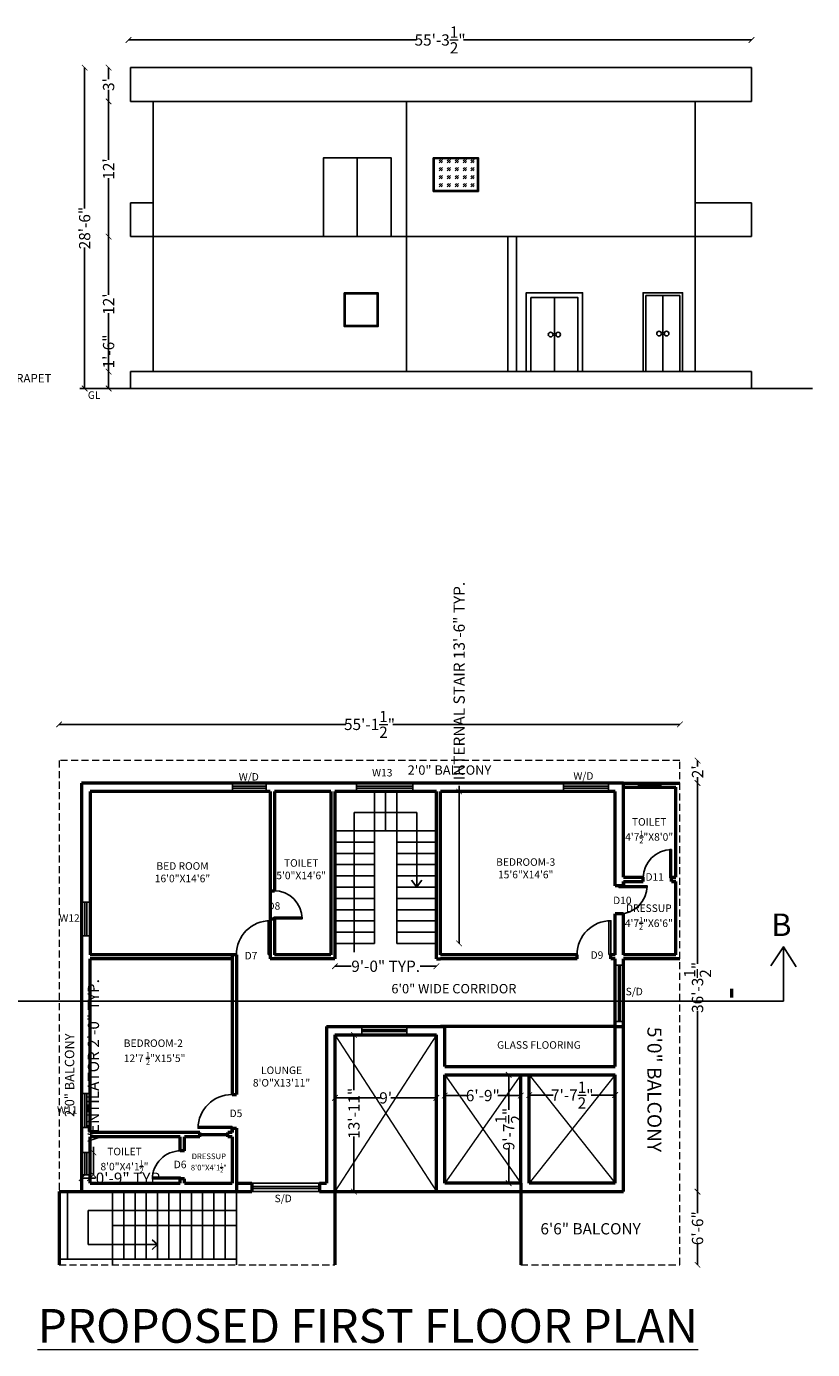
# Model space of a CAD drawing. Units: inches. Extents: x 626 to 5030, y -1681 to 1720.
# Tile 4 of 5: x 3160 to 3997, y 310 to 1720. Entities that reach past the tile are written whole.
import ezdxf
from ezdxf import colors
from ezdxf.entities.mleader import LeaderData, LeaderLine
from ezdxf.math import Vec2, Vec3

# ---------------------------------------------------------------- set-up
doc = ezdxf.new("R2010")
doc.units = ezdxf.units.IN
doc.header["$MEASUREMENT"] = 0
doc.linetypes.add('HIDDENX2', pattern=[0.75, 0.5, -0.25])
for name, color, linetype, lineweight in [('A-ANNO-DIMS', 2, 'Continuous', 18), ('A-ANNO-SYMB', 2, 'Continuous', 25), ('A-ANNO-TEXT', 7, 'Continuous', 18), ('A-AREA-IDEN', 3, 'Continuous', 18), ('A-DOOR', 4, 'Continuous', 25), ('A-ELEV', 7, 'Continuous', 25), ('A-FLOR-OVHD', 3, 'HIDDENX2', 18), ('A-FLOR-PATT', 8, 'Continuous', 18), ('A-FLOR-STRS', 3, 'Continuous', 25), ('A-GLAZ', 4, 'Continuous', 25), ('A-WALL', 7, 'Continuous', 50)]:
    doc.layers.add(name, color=color, linetype=linetype, lineweight=lineweight)
doc.layers.add('windows', color=4, linetype='Continuous')
doc.styles.get("Standard").update_dxf_attribs({"font": 'arial.ttf'})
doc.dimstyles.get("Standard").update_dxf_attribs({"dimtxt": 12, "dimasz": 6, "dimexe": 0.18, "dimexo": 0.0625, "dimgap": 0.09, "dimtad": 0, "dimdec": 1, "dimzin": 0, "dimdsep": 46, "dimlunit": 4, "dimtxsty": 'Standard', "dimblk": 'ARCHTICK', "dimcen": 0.09, "dimse1": 1, "dimse2": 1, "dimclrt": 3, "dimadec": 0, "dimazin": 0, "dimtfac": 1, "dimtdec": 1, "dimtofl": 0, "dimtmove": 0, "dimatfit": 3, "dimfxl": 1, "dimtolj": 1, "dimtzin": 0, "dimarcsym": 0})

# ---------------------------------------------------------------- blocks, each defined once
blk = doc.blocks.new('*U22')
for p, q in [((-750, 0), (-750, -100)), ((0, 0), (0, -100))]:
    blk.add_line(p, q)
blk.add_lwpolyline([(0, 0), (0, 750), (-43.75, 750), (-43.75, 0)], close=True)
blk.add_arc((0, 0), 750, 90, 180)
blk = doc.blocks.new('W3')
at = {"layer": 'windows'}
for p, q in [((2120.1, 414.9), (2120.1, 378.9)), ((2122.1, 414.9), (2122.1, 378.9))]:
    blk.add_line(p, q, dxfattribs=at)
blk.add_lwpolyline([(2116.6, 414.9), (2125.6, 414.9), (2125.6, 378.9), (2116.6, 378.9)], close=True, dxfattribs=at)
blk = doc.blocks.new('W5')
at = {"layer": 'windows'}
for p, q in [((2038.2, 554.9), (2038.2, 494.9)), ((2040.2, 554.9), (2040.2, 494.9))]:
    blk.add_line(p, q, dxfattribs=at)
blk.add_lwpolyline([(2034.7, 554.9), (2043.7, 554.9), (2043.7, 494.9), (2034.7, 494.9)], close=True, dxfattribs=at)
blk = doc.blocks.new('WINDOW')
at = {"layer": 'windows'}
for p, q in [((173.6, 537.5), (173.6, 489.5)), ((175.6, 537.5), (175.6, 489.5))]:
    blk.add_line(p, q, dxfattribs=at)
blk.add_lwpolyline([(170.1, 537.5), (179.1, 537.5), (179.1, 489.5), (170.1, 489.5)], close=True, dxfattribs=at)
blk = doc.blocks.new('*U21')
for p, q in [((0, 0), (0, -100)), ((750, 0), (750, -100))]:
    blk.add_line(p, q)
blk.add_lwpolyline([(0, 0), (0, 750), (43.75, 750), (43.75, 0)], close=True)
blk.add_arc((0, 0), 750, 0, 90)
blk = doc.blocks.new('*U27')
for p, q in [((0, 0), (0, 100)), ((750, 0), (750, 100))]:
    blk.add_line(p, q)
blk.add_lwpolyline([(0, 0), (0, -750), (43.75, -750), (43.75, 0)], close=True)
blk.add_arc((0, 0), 750, 270, 0)
blk = doc.blocks.new('*U28')
for p, q in [((0, 0), (0, -100)), ((750, 0), (750, -100))]:
    blk.add_line(p, q)
blk.add_lwpolyline([(0, 0), (0, 750), (43.75, 750), (43.75, 0)], close=True)
blk.add_arc((0, 0), 750, 0, 90)
blk = doc.blocks.new('_ArchTick')
at = {"color": 0, "linetype": 'ByBlock', "const_width": 0.15}
blk.add_lwpolyline([(-0.5, -0.5), (0.5, 0.5)], dxfattribs=at)
blk = doc.blocks.new('*D29')
at = {"layer": 'A-ANNO-DIMS', "color": 0, "lineweight": -2, "transparency": 16777216}
for p, q in [((3488.3, 578.4), (3536.7, 578.4)), ((3596.3, 578.4), (3547.9, 578.4))]:
    blk.add_line(p, q, dxfattribs=at)
at = {"layer": 'DEFPOINTS', "color": 0, "transparency": 16777216}
for p in [(3596.3, 578.4), (3488.3, 575.4), (3596.3, 562)]:
    blk.add_point(p, dxfattribs=at)
at = {"layer": 'A-ANNO-DIMS', "color": 0, "lineweight": -2, "transparency": 16777216, "xscale": 6, "yscale": 6, "zscale": 6, "rotation": 180}
blk.add_blockref('_ArchTick', (3488.3, 578.4), dxfattribs=at)
at = {"layer": 'A-ANNO-DIMS', "color": 0, "lineweight": -2, "transparency": 16777216, "xscale": 6, "yscale": 6, "zscale": 6}
blk.add_blockref('_ArchTick', (3596.3, 578.4), dxfattribs=at)
at = {"layer": 'A-ANNO-DIMS', "color": 0, "transparency": 16777216, "insert": (3542.3, 578.4), "char_height": 12, "attachment_point": 5}
blk.add_mtext("\\A1;9'", dxfattribs=at)
blk = doc.blocks.new('*D30')
at = {"layer": 'A-ANNO-DIMS', "color": 0, "lineweight": -2, "transparency": 16777216}
for p, q in [((3508.5, 645.5), (3508.5, 586.8)), ((3508.5, 478.5), (3508.5, 537.2))]:
    blk.add_line(p, q, dxfattribs=at)
at = {"layer": 'DEFPOINTS', "color": 0, "transparency": 16777216}
for p in [(3582, 645.5), (3508.5, 478.5), (3582, 478.5)]:
    blk.add_point(p, dxfattribs=at)
at = {"layer": 'A-ANNO-DIMS', "color": 0, "lineweight": -2, "transparency": 16777216, "xscale": 6, "yscale": 6, "zscale": 6}
for p, rotation in [((3508.5, 645.5), 90), ((3508.5, 478.5), 270)]:
    blk.add_blockref('_ArchTick', p, dxfattribs=dict(at, rotation=rotation))
at = {"layer": 'A-ANNO-DIMS', "color": 0, "transparency": 16777216, "insert": (3508.5, 562), "char_height": 12, "attachment_point": 5, "rotation": 90}
blk.add_mtext('\\A1;13\'-11"', dxfattribs=at)
blk = doc.blocks.new('*D31')
at = {"layer": 'A-ANNO-DIMS', "color": 0, "lineweight": -2, "transparency": 16777216}
for p, q in [((3605.3, 580.9), (3629.7, 580.9)), ((3686.3, 580.9), (3661.9, 580.9))]:
    blk.add_line(p, q, dxfattribs=at)
at = {"layer": 'DEFPOINTS', "color": 0, "transparency": 16777216}
for p in [(3605.3, 603), (3686.3, 603), (3686.3, 580.9)]:
    blk.add_point(p, dxfattribs=at)
at = {"layer": 'A-ANNO-DIMS', "color": 0, "lineweight": -2, "transparency": 16777216, "xscale": 6, "yscale": 6, "zscale": 6, "rotation": 180}
blk.add_blockref('_ArchTick', (3605.3, 580.9), dxfattribs=at)
at = {"layer": 'A-ANNO-DIMS', "color": 0, "lineweight": -2, "transparency": 16777216, "xscale": 6, "yscale": 6, "zscale": 6}
blk.add_blockref('_ArchTick', (3686.3, 580.9), dxfattribs=at)
at = {"layer": 'A-ANNO-DIMS', "color": 0, "transparency": 16777216, "insert": (3645.8, 580.9), "char_height": 12, "attachment_point": 5}
blk.add_mtext('\\A1;6\'-9"', dxfattribs=at)
blk = doc.blocks.new('*D32')
at = {"layer": 'A-ANNO-DIMS', "color": 0, "lineweight": -2, "transparency": 16777216}
for p, q in [((3695.3, 581.4), (3720.7, 581.4)), ((3786.8, 581.4), (3761.4, 581.4))]:
    blk.add_line(p, q, dxfattribs=at)
at = {"layer": 'DEFPOINTS', "color": 0, "transparency": 16777216}
for p in [(3695.3, 603), (3786.8, 603), (3786.8, 581.4)]:
    blk.add_point(p, dxfattribs=at)
at = {"layer": 'A-ANNO-DIMS', "color": 0, "lineweight": -2, "transparency": 16777216, "xscale": 6, "yscale": 6, "zscale": 6, "rotation": 180}
blk.add_blockref('_ArchTick', (3695.3, 581.4), dxfattribs=at)
at = {"layer": 'A-ANNO-DIMS', "color": 0, "lineweight": -2, "transparency": 16777216, "xscale": 6, "yscale": 6, "zscale": 6}
blk.add_blockref('_ArchTick', (3786.8, 581.4), dxfattribs=at)
at = {"layer": 'A-ANNO-DIMS', "color": 0, "transparency": 16777216, "insert": (3741.1, 581.4), "char_height": 12, "attachment_point": 5}
blk.add_mtext('\\A1;7\'-7{\\H1x;\\S1/2;}"', dxfattribs=at)
blk = doc.blocks.new('*D33')
at = {"layer": 'A-ANNO-DIMS', "color": 0, "lineweight": -2, "transparency": 16777216}
for p, q in [((3673.4, 603), (3673.4, 565.7)), ((3673.4, 487.5), (3673.4, 524.8))]:
    blk.add_line(p, q, dxfattribs=at)
at = {"layer": 'DEFPOINTS', "color": 0, "transparency": 16777216}
for p in [(3645.8, 603), (3662, 487.5), (3673.4, 487.5)]:
    blk.add_point(p, dxfattribs=at)
at = {"layer": 'A-ANNO-DIMS', "color": 0, "lineweight": -2, "transparency": 16777216, "xscale": 6, "yscale": 6, "zscale": 6}
for p, rotation in [((3673.4, 603), 90), ((3673.4, 487.5), 270)]:
    blk.add_blockref('_ArchTick', p, dxfattribs=dict(at, rotation=rotation))
at = {"layer": 'A-ANNO-DIMS', "color": 0, "transparency": 16777216, "insert": (3673.4, 545.2), "char_height": 12, "attachment_point": 5, "rotation": 90}
blk.add_mtext('\\A1;9\'-7{\\H1x;\\S1/2;}"', dxfattribs=at)
blk = doc.blocks.new('V1')
at = {"layer": 'windows'}
for p, q in [((3301.5, 317.5), (3301.5, 293.5)), ((3303.5, 317.5), (3303.5, 293.5))]:
    blk.add_line(p, q, dxfattribs=at)
blk.add_lwpolyline([(3298, 317.5), (3307, 317.5), (3307, 293.5), (3298, 293.5)], close=True, dxfattribs=at)
blk = doc.blocks.new('*D35')
at = {"layer": 'A-ANNO-DIMS', "color": 0, "lineweight": -2, "transparency": 16777216}
for p, q in [((3194.3, 976.5), (3500, 976.5)), ((3855.8, 976.5), (3550.1, 976.5))]:
    blk.add_line(p, q, dxfattribs=at)
at = {"layer": 'DEFPOINTS', "color": 0, "transparency": 16777216}
for p in [(3194.3, 976.5), (3194.3, 938), (3855.8, 938)]:
    blk.add_point(p, dxfattribs=at)
at = {"layer": 'A-ANNO-DIMS', "color": 0, "lineweight": -2, "transparency": 16777216, "xscale": 6, "yscale": 6, "zscale": 6, "rotation": 180}
blk.add_blockref('_ArchTick', (3194.3, 976.5), dxfattribs=at)
at = {"layer": 'A-ANNO-DIMS', "color": 0, "lineweight": -2, "transparency": 16777216, "xscale": 6, "yscale": 6, "zscale": 6}
blk.add_blockref('_ArchTick', (3855.8, 976.5), dxfattribs=at)
at = {"layer": 'A-ANNO-DIMS', "color": 0, "transparency": 16777216, "insert": (3525.1, 976.5), "char_height": 12, "attachment_point": 5}
blk.add_mtext('\\A1;55\'-1{\\H1x;\\S1/2;}"', dxfattribs=at)
blk = doc.blocks.new('*D36')
at = {"layer": 'A-ANNO-DIMS', "color": 0, "lineweight": -2, "transparency": 16777216}
for p, q in [((3874.6, 938), (3874.6, 931.7)), ((3874.6, 914), (3874.6, 920.3))]:
    blk.add_line(p, q, dxfattribs=at)
at = {"layer": 'DEFPOINTS', "color": 0, "transparency": 16777216}
for p in [(3855.8, 938), (3874.6, 938), (3855.8, 914)]:
    blk.add_point(p, dxfattribs=at)
at = {"layer": 'A-ANNO-DIMS', "color": 0, "lineweight": -2, "transparency": 16777216, "xscale": 6, "yscale": 6, "zscale": 6}
for p, rotation in [((3874.6, 938), 90), ((3874.6, 914), 270)]:
    blk.add_blockref('_ArchTick', p, dxfattribs=dict(at, rotation=rotation))
at = {"layer": 'A-ANNO-DIMS', "color": 0, "transparency": 16777216, "insert": (3874.6, 926), "char_height": 12, "attachment_point": 5, "rotation": 90}
blk.add_mtext("\\A1;2'", dxfattribs=at)
blk = doc.blocks.new('*D37')
at = {"layer": 'A-ANNO-DIMS', "color": 0, "lineweight": -2, "transparency": 16777216}
for p, q in [((3874.6, 914), (3874.6, 721.3)), ((3874.6, 478.5), (3874.6, 671.2))]:
    blk.add_line(p, q, dxfattribs=at)
at = {"layer": 'DEFPOINTS', "color": 0, "transparency": 16777216}
for p in [(3855.8, 914), (3795.8, 478.5), (3874.6, 478.5)]:
    blk.add_point(p, dxfattribs=at)
at = {"layer": 'A-ANNO-DIMS', "color": 0, "lineweight": -2, "transparency": 16777216, "xscale": 6, "yscale": 6, "zscale": 6}
for p, rotation in [((3874.6, 914), 90), ((3874.6, 478.5), 270)]:
    blk.add_blockref('_ArchTick', p, dxfattribs=dict(at, rotation=rotation))
at = {"layer": 'A-ANNO-DIMS', "color": 0, "transparency": 16777216, "insert": (3874.6, 696.2), "char_height": 12, "attachment_point": 5, "rotation": 90}
blk.add_mtext('\\A1;36\'-3{\\H1x;\\S1/2;}"', dxfattribs=at)
blk = doc.blocks.new('*D38')
at = {"layer": 'A-ANNO-DIMS', "color": 0, "lineweight": -2, "transparency": 16777216}
for p, q in [((3874.6, 478.5), (3874.6, 455.6)), ((3874.6, 400.5), (3874.6, 423.4))]:
    blk.add_line(p, q, dxfattribs=at)
at = {"layer": 'DEFPOINTS', "color": 0, "transparency": 16777216}
for p in [(3795.8, 478.5), (3795.8, 400.5), (3874.6, 400.5)]:
    blk.add_point(p, dxfattribs=at)
at = {"layer": 'A-ANNO-DIMS', "color": 0, "lineweight": -2, "transparency": 16777216, "xscale": 6, "yscale": 6, "zscale": 6}
for p, rotation in [((3874.6, 478.5), 90), ((3874.6, 400.5), 270)]:
    blk.add_blockref('_ArchTick', p, dxfattribs=dict(at, rotation=rotation))
at = {"layer": 'A-ANNO-DIMS', "color": 0, "transparency": 16777216, "insert": (3874.6, 439.5), "char_height": 12, "attachment_point": 5, "rotation": 90}
blk.add_mtext('\\A1;6\'-6"', dxfattribs=at)
blk = doc.blocks.new('*D44')
at = {"layer": 'A-ANNO-DIMS', "color": 0, "lineweight": -2, "transparency": 16777216}
for p, q in [((3247.1, 1352.5), (3247.1, 1358.5)), ((3247.1, 1334.5), (3247.1, 1352.5))]:
    blk.add_line(p, q, dxfattribs=at)
at = {"layer": 'DEFPOINTS', "color": 0, "transparency": 16777216}
for p in [(3247.1, 1352.5), (3270.6, 1352.5), (3270.6, 1334.5)]:
    blk.add_point(p, dxfattribs=at)
at = {"layer": 'A-ANNO-DIMS', "color": 0, "lineweight": -2, "transparency": 16777216, "xscale": 6, "yscale": 6, "zscale": 6}
for p, rotation in [((3247.1, 1352.5), 90), ((3247.1, 1334.5), 270)]:
    blk.add_blockref('_ArchTick', p, dxfattribs=dict(at, rotation=rotation))
at = {"layer": 'A-ANNO-DIMS', "color": 0, "transparency": 16777216, "insert": (3247.1, 1374), "char_height": 12, "attachment_point": 5, "rotation": 90}
blk.add_mtext('\\A1;1\'-6"', dxfattribs=at)
blk = doc.blocks.new('*D45')
at = {"layer": 'A-ANNO-DIMS', "color": 0, "lineweight": -2, "transparency": 16777216}
for p, q in [((3247.1, 1496.5), (3247.1, 1434.2)), ((3247.1, 1352.5), (3247.1, 1414.8))]:
    blk.add_line(p, q, dxfattribs=at)
at = {"layer": 'DEFPOINTS', "color": 0, "transparency": 16777216}
for p in [(3247.1, 1496.5), (3270.6, 1496.5), (3270.6, 1352.5)]:
    blk.add_point(p, dxfattribs=at)
at = {"layer": 'A-ANNO-DIMS', "color": 0, "lineweight": -2, "transparency": 16777216, "xscale": 6, "yscale": 6, "zscale": 6}
for p, rotation in [((3247.1, 1496.5), 90), ((3247.1, 1352.5), 270)]:
    blk.add_blockref('_ArchTick', p, dxfattribs=dict(at, rotation=rotation))
at = {"layer": 'A-ANNO-DIMS', "color": 0, "transparency": 16777216, "insert": (3247.1, 1424.5), "char_height": 12, "attachment_point": 5, "rotation": 90}
blk.add_mtext("\\A1;12'", dxfattribs=at)
blk = doc.blocks.new('*D46')
at = {"layer": 'A-ANNO-DIMS', "color": 0, "lineweight": -2, "transparency": 16777216}
for p, q in [((3247.1, 1640.5), (3247.1, 1578.2)), ((3247.1, 1496.5), (3247.1, 1558.8))]:
    blk.add_line(p, q, dxfattribs=at)
at = {"layer": 'DEFPOINTS', "color": 0, "transparency": 16777216}
for p in [(3247.1, 1640.5), (3270.6, 1640.5), (3270.6, 1496.5)]:
    blk.add_point(p, dxfattribs=at)
at = {"layer": 'A-ANNO-DIMS', "color": 0, "lineweight": -2, "transparency": 16777216, "xscale": 6, "yscale": 6, "zscale": 6}
for p, rotation in [((3247.1, 1640.5), 90), ((3247.1, 1496.5), 270)]:
    blk.add_blockref('_ArchTick', p, dxfattribs=dict(at, rotation=rotation))
at = {"layer": 'A-ANNO-DIMS', "color": 0, "transparency": 16777216, "insert": (3247.1, 1568.5), "char_height": 12, "attachment_point": 5, "rotation": 90}
blk.add_mtext("\\A1;12'", dxfattribs=at)
blk = doc.blocks.new('*D47')
at = {"layer": 'A-ANNO-DIMS', "color": 0, "lineweight": -2, "transparency": 16777216}
for p, q in [((3247.1, 1676.5), (3247.1, 1664.1)), ((3247.1, 1640.5), (3247.1, 1652.9))]:
    blk.add_line(p, q, dxfattribs=at)
at = {"layer": 'DEFPOINTS', "color": 0, "transparency": 16777216}
for p in [(3247.1, 1676.5), (3270.6, 1676.5), (3270.6, 1640.5)]:
    blk.add_point(p, dxfattribs=at)
at = {"layer": 'A-ANNO-DIMS', "color": 0, "lineweight": -2, "transparency": 16777216, "xscale": 6, "yscale": 6, "zscale": 6}
for p, rotation in [((3247.1, 1676.5), 90), ((3247.1, 1640.5), 270)]:
    blk.add_blockref('_ArchTick', p, dxfattribs=dict(at, rotation=rotation))
at = {"layer": 'A-ANNO-DIMS', "color": 0, "transparency": 16777216, "insert": (3247.1, 1658.5), "char_height": 12, "attachment_point": 5, "rotation": 90}
blk.add_mtext("\\A1;3'", dxfattribs=at)
blk = doc.blocks.new('*D48')
at = {"layer": 'A-ANNO-DIMS', "color": 0, "lineweight": -2, "transparency": 16777216}
for p, q in [((3221.6, 1676.5), (3221.6, 1526.3)), ((3221.6, 1334.5), (3221.6, 1484.7))]:
    blk.add_line(p, q, dxfattribs=at)
at = {"layer": 'DEFPOINTS', "color": 0, "transparency": 16777216}
for p in [(3270.6, 1676.5), (3221.6, 1334.5), (3270.6, 1334.5)]:
    blk.add_point(p, dxfattribs=at)
at = {"layer": 'A-ANNO-DIMS', "color": 0, "lineweight": -2, "transparency": 16777216, "xscale": 6, "yscale": 6, "zscale": 6}
for p, rotation in [((3221.6, 1676.5), 90), ((3221.6, 1334.5), 270)]:
    blk.add_blockref('_ArchTick', p, dxfattribs=dict(at, rotation=rotation))
at = {"layer": 'A-ANNO-DIMS', "color": 0, "transparency": 16777216, "insert": (3221.6, 1505.5), "char_height": 12, "attachment_point": 5, "rotation": 90}
blk.add_mtext('\\A1;28\'-6"', dxfattribs=at)
blk = doc.blocks.new('*D50')
at = {"layer": 'A-ANNO-DIMS', "color": 0, "lineweight": -2, "transparency": 16777216}
for p, q in [((3268.4, 1706), (3575.2, 1706)), ((3932.1, 1706), (3625.4, 1706))]:
    blk.add_line(p, q, dxfattribs=at)
at = {"layer": 'DEFPOINTS', "color": 0, "transparency": 16777216}
for p in [(3932.1, 1706), (3268.4, 1676.5), (3932.1, 1676.5)]:
    blk.add_point(p, dxfattribs=at)
at = {"layer": 'A-ANNO-DIMS', "color": 0, "lineweight": -2, "transparency": 16777216, "xscale": 6, "yscale": 6, "zscale": 6, "rotation": 180}
blk.add_blockref('_ArchTick', (3268.4, 1706), dxfattribs=at)
at = {"layer": 'A-ANNO-DIMS', "color": 0, "lineweight": -2, "transparency": 16777216, "xscale": 6, "yscale": 6, "zscale": 6}
blk.add_blockref('_ArchTick', (3932.1, 1706), dxfattribs=at)
at = {"layer": 'A-ANNO-DIMS', "color": 0, "transparency": 16777216, "insert": (3600.3, 1706), "char_height": 12, "attachment_point": 5}
blk.add_mtext('\\A1;55\'-3{\\H1x;\\S1/2;}"', dxfattribs=at)
blk = doc.blocks.new('STAIR-INTERNAL')
for p, q in [((42, 120), (42, 162)), ((54, 120), (54, 162)), ((66, 120), (66, 162)), ((20.4, 139.7), (87.3, 139.7)), ((87.3, 139.7), (87.3, 60)), ((108, 120), (0, 120)), ((0, 120), (42, 120)), ((42, 120), (42, 0)), ((66, 0), (66, 120)), ((0, 108), (42, 108)), ((108, 108), (66, 108)), ((0, 96), (42, 96)), ((108, 96), (66, 96)), ((0, 84), (42, 84)), ((0, 72), (42, 72)), ((108, 84), (66, 84)), ((108, 72), (66, 72)), ((0, 60), (42, 60)), ((108, 60), (66, 60)), ((87.3, 60), (81.6, 67.5)), ((86.7, 60), (92.4, 67.5)), ((0, 48), (42, 48)), ((108, 48), (66, 48)), ((0, 36), (42, 36)), ((108, 36), (66, 36)), ((0, 24), (42, 24)), ((108, 24), (66, 24)), ((0, 12), (42, 12)), ((108, 12), (66, 12)), ((0, 0), (42, 0)), ((108, 0), (66, 0))]:
    blk.add_line(p, q)
blk = doc.blocks.new('STAIR-ENTRANCE')
for p, q in [((26.1, 78), (26.1, 0)), ((38.1, 78), (38.1, 6)), ((50.1, 78), (50.1, 6)), ((62.1, 78), (62.1, 6)), ((74.1, 78), (74.1, 6)), ((86.1, 78), (86.1, 6)), ((98.1, 78), (98.1, 6)), ((110.1, 78), (110.1, 6)), ((122.1, 78), (122.1, 6)), ((134.1, 78), (134.1, 6)), ((146.1, 78), (146.1, 6)), ((158.1, 78), (158.1, 0)), ((158.1, 57.8), (0, 57.8)), ((0, 57.8), (0, 21.7)), ((26.1, 42), (158.1, 42)), ((0, 21.7), (74.1, 21.7)), ((74.1, 21.7), (68.4, 26.8)), ((74.1, 21.7), (68.4, 16.5))]:
    blk.add_line(p, q)
blk = doc.blocks.new('*D60')
at = {"layer": 'A-ANNO-DIMS', "color": 0, "lineweight": -2, "transparency": 16777216}
for p, q in [((3230.9, 520.4), (3230.9, 526.4)), ((3230.9, 496.4), (3230.9, 520.4))]:
    blk.add_line(p, q, dxfattribs=at)
at = {"layer": 'DEFPOINTS', "color": 0, "transparency": 16777216}
for p in [(3227.3, 520.4), (3230.9, 520.4), (3227.3, 496.4)]:
    blk.add_point(p, dxfattribs=at)
at = {"layer": 'A-ANNO-DIMS', "color": 0, "lineweight": -2, "transparency": 16777216, "xscale": 6, "yscale": 6, "zscale": 6}
for p, rotation in [((3230.9, 520.4), 90), ((3230.9, 496.4), 270)]:
    blk.add_blockref('_ArchTick', p, dxfattribs=dict(at, rotation=rotation))
at = {"layer": 'A-ANNO-DIMS', "color": 3, "transparency": 16777216, "insert": (3230.9, 618.3), "char_height": 12, "attachment_point": 5, "rotation": 90}
blk.add_mtext('\\A1;VENTILATOR 2\'-0" TYP.', dxfattribs=at)
blk = doc.blocks.new('*D61')
at = {"layer": 'A-ANNO-DIMS', "color": 0, "lineweight": -2, "transparency": 16777216}
for p, q in [((3218.3, 492.8), (3227.3, 492.8)), ((3227.3, 492.8), (3233.3, 492.8))]:
    blk.add_line(p, q, dxfattribs=at)
at = {"layer": 'DEFPOINTS', "color": 0, "transparency": 16777216}
for p in [(3218.3, 496.4), (3227.3, 496.4), (3227.3, 492.8)]:
    blk.add_point(p, dxfattribs=at)
at = {"layer": 'A-ANNO-DIMS', "color": 0, "lineweight": -2, "transparency": 16777216, "xscale": 6, "yscale": 6, "zscale": 6, "rotation": 180}
blk.add_blockref('_ArchTick', (3218.3, 492.8), dxfattribs=at)
at = {"layer": 'A-ANNO-DIMS', "color": 0, "lineweight": -2, "transparency": 16777216, "xscale": 6, "yscale": 6, "zscale": 6}
blk.add_blockref('_ArchTick', (3227.3, 492.8), dxfattribs=at)
at = {"layer": 'A-ANNO-DIMS', "color": 3, "transparency": 16777216, "insert": (3270, 492.8), "char_height": 12, "attachment_point": 5}
blk.add_mtext('\\A1;0\'-9" TYP.', dxfattribs=at)
blk = doc.blocks.new('*D62')
at = {"layer": 'A-ANNO-DIMS', "color": 0, "lineweight": -2, "transparency": 16777216}
for p, q in [((3620.6, 905), (3620.6, 911)), ((3620.6, 743), (3620.6, 905))]:
    blk.add_line(p, q, dxfattribs=at)
at = {"layer": 'DEFPOINTS', "color": 0, "transparency": 16777216}
for p in [(3596.3, 905), (3620.6, 905), (3596.3, 743)]:
    blk.add_point(p, dxfattribs=at)
at = {"layer": 'A-ANNO-DIMS', "color": 0, "lineweight": -2, "transparency": 16777216, "xscale": 6, "yscale": 6, "zscale": 6}
for p, rotation in [((3620.6, 905), 90), ((3620.6, 743), 270)]:
    blk.add_blockref('_ArchTick', p, dxfattribs=dict(at, rotation=rotation))
at = {"layer": 'A-ANNO-DIMS', "color": 3, "transparency": 16777216, "insert": (3620.6, 1022.7), "char_height": 12, "attachment_point": 5, "rotation": 90}
blk.add_mtext('\\A1;INTERNAL STAIR 13\'-6" TYP.', dxfattribs=at)
blk = doc.blocks.new('*D63')
at = {"layer": 'A-ANNO-DIMS', "color": 0, "lineweight": -2, "transparency": 16777216}
for p, q in [((3488.3, 718.7), (3505.6, 718.7)), ((3596.3, 718.7), (3579, 718.7))]:
    blk.add_line(p, q, dxfattribs=at)
at = {"layer": 'DEFPOINTS', "color": 0, "transparency": 16777216}
for p in [(3488.3, 743), (3596.3, 743), (3596.3, 718.7)]:
    blk.add_point(p, dxfattribs=at)
at = {"layer": 'A-ANNO-DIMS', "color": 0, "lineweight": -2, "transparency": 16777216, "xscale": 6, "yscale": 6, "zscale": 6, "rotation": 180}
blk.add_blockref('_ArchTick', (3488.3, 718.7), dxfattribs=at)
at = {"layer": 'A-ANNO-DIMS', "color": 0, "lineweight": -2, "transparency": 16777216, "xscale": 6, "yscale": 6, "zscale": 6}
blk.add_blockref('_ArchTick', (3596.3, 718.7), dxfattribs=at)
at = {"layer": 'A-ANNO-DIMS', "color": 3, "transparency": 16777216, "insert": (3542.3, 718.7), "char_height": 12, "attachment_point": 5}
blk.add_mtext('\\A1;9\'-0" TYP.', dxfattribs=at)

msp = doc.modelspace()

# ---------------------------------------------------------------- hatches: boundary and pattern name
at = {"layer": 'A-GLAZ'}
h = msp.add_hatch(dxfattribs=at)
h.set_pattern_fill('GOST_GLASS', color=256)
h.set_pattern_definition([(45, (-49.396, -487), (8.485281, 0), [5, -7]), (45, (-47.275, -487), (8.485281, 0), [2, -10]), (45, (-49.396, -484.8787), (8.485281, 0), [2, -10])])
h.paths.add_polyline_path([(3640.08, 1545.5), (3640.08, 1579.5), (3594.08, 1579.5), (3594.08, 1545.5)])

# ---------------------------------------------------------------- linework, layer by layer
at = {"layer": 'A-ANNO-SYMB'}
for p, q in [((3966.1, 681.5), (3966.1, 739.5)), ((2128.1, 681.5), (3966.1, 681.5))]:
    msp.add_line(p, q, dxfattribs=at)
msp.add_lwpolyline([(3952.6, 719), (3966.1, 739.5), (3979.6, 718)], dxfattribs=at)
at = {"layer": 'A-DOOR'}
for p, q in [((3790.3, 720), (3790.3, 660)), ((3792.3, 720), (3792.3, 660)), ((3399.8, 484), (3471.8, 484)), ((3399.8, 482), (3471.8, 482))]:
    msp.add_line(p, q, dxfattribs=at)
for points in [[(3786.8, 720), (3795.8, 720), (3795.8, 660), (3786.8, 660)], [(3399.8, 478.5), (3399.8, 487.5), (3471.8, 487.5), (3471.8, 478.5)]]:
    msp.add_lwpolyline(points, close=True, dxfattribs=at)
at = {"layer": 'A-ELEV'}
for p, q in [((3270.6, 1640.5), (3270.6, 1676.5)), ((3270.6, 1676.5), (3932.1, 1676.5)), ((3932.1, 1640.5), (3932.1, 1676.5)), ((3270.6, 1640.5), (3932.1, 1640.5)), ((3294.6, 1352.5), (3294.6, 1640.5)), ((3564.6, 1352.5), (3564.6, 1640.5)), ((3872.1, 1352.5), (3872.1, 1640.5)), ((3294.6, 1496.5), (3294.6, 1634.5)), ((3872.1, 1496.5), (3872.1, 1634.5)), ((3512.1, 1580.5), (3512.1, 1496.5)), ((3270.6, 1496.5), (3270.6, 1532.5)), ((3270.6, 1532.5), (3294.6, 1532.5)), ((3927.6, 1532.5), (3872.1, 1532.5)), ((3927.6, 1532.5), (3932.1, 1532.5)), ((3932.1, 1496.5), (3932.1, 1532.5)), ((3270.6, 1496.5), (3932.1, 1496.5)), ((3672.6, 1352.5), (3672.6, 1496.5)), ((3681.6, 1352.5), (3681.6, 1496.5)), ((3294.6, 1352.5), (3294.6, 1490.5)), ((3872.1, 1352.5), (3872.1, 1490.5)), ((3722.1, 1431.5), (3722.1, 1352.5)), ((3837.6, 1433.5), (3837.6, 1352.5)), ((3270.6, 1334.5), (3270.6, 1352.5)), ((3270.6, 1352.5), (3932.1, 1352.5)), ((3932.1, 1334.5), (3932.1, 1352.5)), ((3216.6, 1334.5), (3997.1, 1334.5))]:
    msp.add_line(p, q, dxfattribs=at)
for points in [[(3476.1, 1496.5), (3476.1, 1580.5), (3548.1, 1580.5), (3548.1, 1496.5)], [(3692.1, 1352.5), (3692.1, 1436.5), (3752.1, 1436.5), (3752.1, 1352.5)], [(3697.1, 1352.5), (3697.1, 1431.5), (3747.1, 1431.5), (3747.1, 1352.5)], [(3816.6, 1352.5), (3816.6, 1436.5), (3858.6, 1436.5), (3858.6, 1352.5)], [(3819.6, 1352.5), (3819.6, 1433.5), (3855.6, 1433.5), (3855.6, 1352.5)]]:
    msp.add_lwpolyline(points, dxfattribs=at)
for points in [[(3593.08, 1580.5), (3641.08, 1580.5), (3641.08, 1544.5), (3593.08, 1544.5)], [(3594.08, 1579.5), (3640.08, 1579.5), (3640.08, 1545.5), (3594.08, 1545.5)], [(3498.23, 1436.5), (3534.23, 1436.5), (3534.23, 1400.5), (3498.23, 1400.5)], [(3499.23, 1435.5), (3533.23, 1435.5), (3533.23, 1401.5), (3499.23, 1401.5)]]:
    msp.add_lwpolyline(points, close=True, dxfattribs=at)
for centre in [(3718.1, 1392), (3726.1, 1392), (3833.6, 1393), (3841.6, 1393)]:
    msp.add_circle(centre, 2.5, dxfattribs=at)
at = {"layer": 'A-FLOR-OVHD', "ltscale": 15}
msp.add_lwpolyline([(3686.3, 400.5), (3855.8, 400.5), (3855.8, 938), (3194.3, 938), (3194.3, 400.5), (3407.3, 400.5), (3488.3, 400.5)], dxfattribs=at)
at = {"layer": 'A-FLOR-PATT'}
for p, q in [((3488.3, 645.5), (3596.3, 478.5)), ((3596.3, 645.5), (3488.3, 478.5)), ((3605.3, 603), (3686.3, 487.5)), ((3686.3, 603), (3605.3, 487.5)), ((3695.3, 603), (3786.8, 487.5)), ((3786.8, 603), (3695.3, 487.5))]:
    msp.add_line(p, q, dxfattribs=at)
at = {"layer": 'A-FLOR-STRS'}
for p, q in [((3508.69, 733.76), (3508.69, 882.68)), ((3203.3, 478.5), (3203.3, 406.5)), ((3194.3, 406.5), (3383.3, 406.5))]:
    msp.add_line(p, q, dxfattribs=at)
at = {"layer": 'A-GLAZ'}
msp.add_line((3811.55, 911.75), (3835.55, 911.75), dxfattribs=at)
msp.add_lwpolyline([(3811.55, 909.5), (3811.55, 914), (3835.55, 914), (3835.55, 909.5)], close=True, dxfattribs=at)
at = {"layer": 'A-WALL'}
for p, q in [((3795.8, 914), (3218.3, 914)), ((3218.3, 914), (3218.3, 478.5)), ((3419.3, 905), (3227.3, 905)), ((3227.3, 905), (3227.3, 731)), ((3419.3, 905), (3419.3, 726.5)), ((3483.8, 905), (3423.8, 905)), ((3423.8, 905), (3423.8, 799.22)), ((3483.8, 905), (3483.8, 731)), ((3596.3, 905), (3488.3, 905)), ((3488.3, 905), (3488.3, 726.5)), ((3596.3, 726.5), (3596.3, 905)), ((3786.8, 905), (3600.8, 905)), ((3600.8, 731), (3600.8, 905)), ((3786.8, 804.5), (3786.8, 905)), ((3795.8, 914), (3855.8, 914)), ((3795.8, 813.5), (3795.8, 914)), ((3795.8, 909.5), (3851.3, 909.5)), ((3851.3, 813.5), (3851.3, 909.5)), ((3795.8, 804.5), (3786.8, 804.5)), ((3795.8, 813.5), (3816.8, 813.5)), ((3795.8, 809), (3816.8, 809)), ((3795.8, 809), (3795.8, 804.5)), ((3795.8, 804.5), (3795.8, 809)), ((3816.8, 809), (3816.8, 813.5)), ((3846.8, 809), (3846.8, 813.5)), ((3846.8, 813.5), (3851.3, 813.5)), ((3851.3, 809), (3846.8, 809)), ((3846.8, 809), (3851.3, 809)), ((3851.3, 731), (3851.3, 809)), ((3419.3, 799.22), (3419.3, 731)), ((3419.3, 799.22), (3423.8, 799.22)), ((3419.3, 769.22), (3423.8, 769.22)), ((3423.8, 769.22), (3423.8, 731)), ((3795.8, 774.5), (3786.8, 774.5)), ((3786.8, 731), (3786.8, 774.5)), ((3795.8, 731), (3795.8, 774.5)), ((3383.3, 731), (3227.3, 731)), ((3378.8, 726.5), (3227.3, 726.5)), ((3378.8, 731), (3378.8, 726.5)), ((3378.8, 726.5), (3378.8, 582)), ((3383.3, 731), (3383.3, 582)), ((3488.3, 726.5), (3419.3, 726.5)), ((3483.8, 731), (3423.8, 731)), ((3596.3, 726.5), (3600.8, 726.5)), ((3746.3, 731), (3600.8, 731)), ((3746.3, 726.5), (3600.8, 726.5)), ((3746.3, 726.5), (3746.3, 731)), ((3786.8, 731), (3782.3, 731)), ((3782.3, 726.5), (3782.3, 731)), ((3786.8, 726.5), (3782.3, 726.5)), ((3786.8, 726.5), (3782.3, 726.5)), ((3786.8, 612), (3786.8, 726.5)), ((3851.3, 731), (3795.8, 731)), ((3795.8, 478.5), (3795.8, 726.5)), ((3855.8, 726.5), (3795.8, 726.5)), ((3910.8, 694.5), (3910.8, 685.5)), ((3479.3, 654.5), (3479.3, 487.5)), ((3479.3, 654.5), (3605.3, 654.5)), ((3786.8, 654.5), (3600.8, 654.5)), ((3605.3, 612), (3605.3, 654.5)), ((3786.8, 654.5), (3795.8, 654.5)), ((3488.3, 645.5), (3488.3, 400.5)), ((3488.3, 645.5), (3596.3, 645.5)), ((3596.3, 478.5), (3596.3, 645.5)), ((3605.3, 612), (3786.8, 612)), ((3605.3, 603), (3686.3, 603)), ((3605.3, 487.5), (3605.3, 603)), ((3675.8, 603), (3686.3, 603)), ((3686.3, 487.5), (3686.3, 603)), ((3686.3, 603), (3786.8, 603)), ((3695.3, 487.5), (3695.3, 603)), ((3786.8, 487.5), (3786.8, 603)), ((3378.8, 582), (3383.3, 582)), ((3344.3, 541.5), (3227.3, 541.5)), ((3323.3, 537), (3227.3, 537)), ((3344.3, 537), (3327.8, 537)), ((3344.3, 537), (3344.3, 541.5)), ((3344.3, 539.25), (3374.3, 539.25)), ((3378.8, 541.5), (3374.3, 541.5)), ((3374.3, 537), (3374.3, 541.5)), ((3378.8, 537), (3374.3, 537)), ((3378.8, 537), (3374.3, 537)), ((3378.8, 541.5), (3378.8, 546)), ((3378.8, 546), (3383.3, 546)), ((3378.8, 546), (3378.8, 541.5)), ((3378.8, 537), (3378.8, 487.5)), ((3383.3, 546), (3383.3, 478.5)), ((3327.8, 522), (3323.3, 522)), ((3227.3, 487.5), (3323.3, 487.5)), ((3327.8, 492), (3323.3, 492)), ((3327.8, 487.5), (3378.8, 487.5)), ((3383.3, 487.5), (3399.8, 487.5)), ((3399.8, 487.5), (3399.8, 478.5)), ((3471.8, 487.5), (3471.8, 478.5)), ((3471.8, 487.5), (3479.3, 487.5)), ((3686.3, 487.5), (3605.3, 487.5)), ((3686.3, 487.5), (3686.3, 400.5)), ((3786.8, 487.5), (3695.3, 487.5)), ((3194.3, 478.5), (3399.8, 478.5)), ((3194.3, 478.5), (3194.3, 400.5)), ((3471.8, 478.5), (3488.3, 478.5)), ((3488.3, 478.5), (3596.3, 478.5)), ((3596.3, 478.5), (3795.8, 478.5)), ((3686.3, 478.5), (3795.8, 478.5)), ((3782.3, 478.5), (3795.8, 478.5))]:
    msp.add_line(p, q, dxfattribs=at)
for points in [[(3227.3, 541.5), (3227.3, 546.92), (3227.3, 582.92), (3227.3, 726.5)], [(3227.3, 487.5), (3227.3, 537)], [(3323.3, 522), (3323.3, 537)], [(3327.8, 522), (3327.8, 537)], [(3323.3, 487.5), (3323.3, 492)], [(3327.8, 487.5), (3327.8, 492)]]:
    msp.add_lwpolyline(points, dxfattribs=at)

# ---------------------------------------------------------------- block references
at = {"layer": 'A-DOOR'}
for name, p, xscale, yscale, zscale in [('*U21', (3846.8, 813), -0.04, 0.04, 0.04), ('*U22', (3419.3, 731.3), 0.0479999999999998, 0.0479999999999998, 0.0479999999999998), ('*U22', (3782.3, 731.3), 0.0479999999999998, 0.0479999999999998, 0.0479999999999998)]:
    msp.add_blockref(name, p, dxfattribs=dict(at, xscale=xscale, yscale=yscale, zscale=zscale))
for name, p, xscale, yscale, zscale, rotation in [('*U22', (3790.8, 804.5), -0.04, 0.04, 0.04, 270), ('*U21', (3423.3, 769.22), -0.04, 0.04, 0.04, 270), ('*U28', (3378.5, 546), 0.0479999999999998, 0.0479999999999998, 0.0479999999999998, 90), ('*U27', (3323.8, 492), -0.04, 0.04, 0.04, 270)]:
    msp.add_blockref(name, p, dxfattribs=dict(at, xscale=xscale, yscale=yscale, zscale=zscale, rotation=rotation))
at = {"layer": 'A-FLOR-STRS'}
for name, p in [('STAIR-INTERNAL', (3488.3, 743)), ('STAIR-ENTRANCE', (3225.16, 400.5))]:
    msp.add_blockref(name, p, dxfattribs=at)
at = {"layer": 'A-GLAZ', "rotation": 90}
for name, p in [('W3', (3793.87, -1211.6)), ('W5', (4066.22, -1129.66)), ('WINDOW', (4269.13, 734.95)), ('WINDOW', (4054.3, 475.45))]:
    msp.add_blockref(name, p, dxfattribs=at)
at = {"layer": 'A-GLAZ'}
for name, p in [('W3', (1101.7, 372.13)), ('W3', (1101.7, 168.05)), ('V1', (-79.7, 202.87))]:
    msp.add_blockref(name, p, dxfattribs=at)

# ---------------------------------------------------------------- texts
at = {"layer": 'A-ANNO-SYMB', "insert": (3947.97, 774.94), "char_height": 24, "attachment_point": 1}
msp.add_mtext_dynamic_manual_height_columns('\\pxqc;B ', width=31.8381, gutter_width=1, heights=[0], dxfattribs=at)
at = {"layer": 'A-ANNO-TEXT', "attachment_point": 1}
for s, width, insert, char_height in [('\\pxqc;GL', 31.8381, (3215.77, 1331.5), 8), ('\\pxqc;2\'0" BALCONY', 192.2401, (3514.15, 932.85), 10), ('\\pxqc;W/D', 31.8381, (3380.56, 924.59), 8), ('\\pxqc;W13', 31.8381, (3522.77, 929), 8), ('\\pxqc;W/D', 31.8381, (3737.06, 925.59), 8), ('\\pxqc;D11', 38.7401, (3809.6, 817.91), 8), ('\\pxqc;D10', 38.7401, (3775.1, 792.91), 8), ('\\pxqc;D8', 38.7401, (3403.86, 787), 8), ('\\pxqc;W12', 31.8381, (3189.56, 774.09), 8), ('\\pxqc;D7', 38.7401, (3379.43, 733.97), 8), ('\\pxqc;D9', 38.7401, (3748.06, 734.67), 8), ('\\pxqc;6\'0" WIDE CORRIDOR', 246.7279, (3491.64, 699.81), 10), ('\\pxqc;S/D', 38.7401, (3787.8, 695.77), 8), ('\\pxqc;GLASS FLOORING', 246.7279, (3582.25, 638.82), 8), ('\\pxqc;W11', 31.8381, (3187.06, 569.59), 8), ('\\pxqc;D5', 38.7401, (3363.43, 565.97), 8), ('\\pxqc;D6', 38.7401, (3303.93, 511.47), 8), ('\\pxqc;S/D', 38.7401, (3413.76, 475.24), 8), ('\\pxqc;6\'6" BALCONY', 192.2401, (3664.53, 444.9), 12), ('\\pxt25;{\\LPROPOSED FIRST FLOOR PLAN}', 941.0725, (3171.53, 353.4), 36)]:
    msp.add_mtext_dynamic_manual_height_columns(s, width=width, gutter_width=1, heights=[0], dxfattribs=dict(at, insert=insert, char_height=char_height))
for s, insert, char_height, rotation in [('\\pxqc;5\'0" BALCONY', (3836.18, 683.46), 15, 270), ('\\pxqc;2\'0" BALCONY', (3200.52, 506.48), 10, 90)]:
    msp.add_mtext_dynamic_manual_height_columns(s, width=192.2401, gutter_width=1, heights=[0], dxfattribs=dict(at, insert=insert, char_height=char_height, rotation=rotation))
at = {"layer": 'A-AREA-IDEN', "attachment_point": 1}
for s, width, insert, char_height in [('\\A1;\\pxqc;TOILET\\P4\'7{\\H0.7x;\\S1/2;}"X8\'0"', 60.9983, (3792.56, 876.58), 8), ('\\pxqc;TOILET\\P5\'0"X14\'6"', 100.5461, (3402.03, 832.81), 8), ('\\pxqc;BEDROOM-3\\P15\'6"X14\'6"', 100.5461, (3641.24, 833.77), 8), ('\\pxqc;BED ROOM\\P16\'0"X14\'6"', 100.5461, (3275.57, 829.6), 8), ('\\A1;\\pxqc;DRESSUP\\P4\'7{\\H0.7x;\\S1/2;}"X6\'6"', 60.9983, (3792.22, 784.62), 8), ('\\A1;BEDROOM-2\\P12\'7 {\\H0.7x;\\S1/2;}"X15\'5"', 70.7738, (3263.26, 640.72), 8), ('\\A1;\\pxqc;LOUNGE\\P8\'O"X13\'11"', 70.7738, (3395.98, 611.85), 8), ('\\A1;\\pxqc;TOILET\\P8\'0"X4\'1{\\H0.7x;\\S1/2;}"', 60.9983, (3233.53, 525.23), 8), ('\\A1;\\pxqc;DRESSUP\\P8\'0"X4\'1{\\H0.7x;\\S1/2;}"', 60.9983, (3323.39, 519.14), 6)]:
    msp.add_mtext_dynamic_manual_height_columns(s, width=width, gutter_width=1, heights=[0], dxfattribs=dict(at, insert=insert, char_height=char_height))

# ---------------------------------------------------------------- dimensions: what is measured, and where the dimension line sits
at = {"layer": 'A-ANNO-DIMS'}
for base, p1, p2, picture, middle in [((3932.1039, 1706), (3268.4495, 1676.5), (3932.1039, 1676.5), '*D50', (3600.2767, 1706)), ((3194.3, 976.5), (3855.8, 938), (3194.3, 938), '*D35', (3525.05, 976.5)), ((3686.3, 580.95), (3605.3, 603), (3686.3, 603), '*D31', (3645.8, 580.95)), ((3786.8, 581.4), (3695.3, 603), (3786.8, 603), '*D32', (3741.05, 581.4)), ((3596.3, 578.4), (3488.3, 575.4), (3596.3, 562), '*D29', (3542.3, 578.4))]:
    dim = msp.add_linear_dim(base=base, p1=p1, p2=p2, dimstyle='Standard', override={"dimclrd": 0, "dimclre": 0, "dimclrt": 0}, dxfattribs=at)
    dim.commit()
    dim.dimension.update_dxf_attribs({"geometry": picture, "text_midpoint": middle})
for base, p1, p2, picture, middle in [((3221.6, 1334.5), (3270.6, 1676.5), (3270.6, 1334.5), '*D48', (3221.6, 1505.5)), ((3247.1, 1676.5), (3270.6, 1640.5), (3270.6, 1676.5), '*D47', (3247.1, 1658.5)), ((3247.1, 1640.5), (3270.6, 1496.5), (3270.6, 1640.5), '*D46', (3247.1, 1568.5)), ((3247.1, 1496.5), (3270.6, 1352.5), (3270.6, 1496.5), '*D45', (3247.1, 1424.5)), ((3247.1, 1352.5), (3270.6, 1334.5), (3270.6, 1352.5), '*D44', (3247.1, 1373.97)), ((3874.6, 938), (3855.8, 914), (3855.8, 938), '*D36', (3874.6, 926)), ((3874.6, 478.5), (3855.8, 914), (3795.8, 478.5), '*D37', (3874.6, 696.25)), ((3508.48, 478.5), (3581.98, 645.5), (3581.98, 478.5), '*D30', (3508.48, 562)), ((3673.35, 487.5), (3645.8, 603), (3661.98, 487.5), '*D33', (3673.35, 545.25)), ((3874.6, 400.5), (3795.8, 478.5), (3795.8, 400.5), '*D38', (3874.6, 439.5))]:
    dim = msp.add_linear_dim(base=base, p1=p1, p2=p2, angle=90, dimstyle='Standard', override={"dimclrd": 0, "dimclre": 0, "dimclrt": 0}, dxfattribs=at)
    dim.commit()
    dim.dimension.update_dxf_attribs({"geometry": picture, "text_midpoint": middle})
for base, p1, p2, text, picture, middle in [((3620.6, 905), (3596.3, 743), (3596.3, 905), 'INTERNAL STAIR <> TYP.', '*D62', (3620.6, 1022.68)), ((3230.9, 520.4), (3227.3, 496.4), (3227.3, 520.4), 'VENTILATOR <> TYP.', '*D60', (3230.9, 618.33))]:
    dim = msp.add_linear_dim(base=base, p1=p1, p2=p2, angle=90, text=text, dimstyle='Standard', override={"dimdec": 1, "dimrnd": 0, "dimzin": 1, "dimlunit": 4, "dimfrac": 2}, dxfattribs=at)
    dim.commit()
    dim.dimension.update_dxf_attribs({"geometry": picture, "text_midpoint": middle})
for base, p1, p2, picture, middle in [((3596.3, 718.7), (3488.3, 743), (3596.3, 743), '*D63', (3542.3, 718.7)), ((3227.3, 492.8), (3218.3, 496.4), (3227.3, 496.4), '*D61', (3269.96, 492.8))]:
    dim = msp.add_linear_dim(base=base, p1=p1, p2=p2, text='<> TYP.', dimstyle='Standard', override={"dimdec": 1, "dimrnd": 0, "dimzin": 1, "dimlunit": 4, "dimfrac": 2}, dxfattribs=at)
    dim.commit()
    dim.dimension.update_dxf_attribs({"geometry": picture, "text_midpoint": middle})

# ---------------------------------------------------------------- leaders
at = {"layer": 'A-ANNO-TEXT'}
ml = msp.add_multileader_mtext('Standard', dxfattribs=at)
ml.set_content('PLINTH LEVELPARAPET', color=256)
ml.set_leader_properties()
ml.build(insert=Vec2(0, 0))
ml.multileader.update_dxf_attribs({"dogleg_length": 0.36, "arrow_head_size": 0.18})
ctx = ml.context
ctx.base_point, ctx.char_height, ctx.arrow_head_size, ctx.landing_gap_size, ctx.plane_origin = Vec3(3052.46, 1345.5), 9, 0.18, 0.09, Vec3(3013.6, 1345.5)
notes = []
notes.append((ctx, [(0, (1, 1, 0), (3052.1, 1345.5), (1, 0), 0.36, [(0, [(3013.6, 1345.5)], 0, [])])]))
ctx.mtext.insert, ctx.mtext.flow_direction = Vec3(3052.55, 1350), 5
for ctx, leaders in notes:
    for number, flags, end, landing, length, lines in leaders:
        leader = LeaderData()
        leader.index, (leader.has_last_leader_line, leader.has_dogleg_vector, leader.attachment_direction) = number, flags
        leader.last_leader_point, leader.dogleg_vector, leader.dogleg_length = Vec3(end), Vec3(landing), length
        for number, points, colour, breaks in lines:
            line = LeaderLine()
            line.index, line.vertices, line.color, line.breaks = number, Vec3.list(points), colors.encode_raw_color(colour), breaks
            leader.lines.append(line)
        ctx.leaders.append(leader)

doc.saveas('drawing.dxf')
